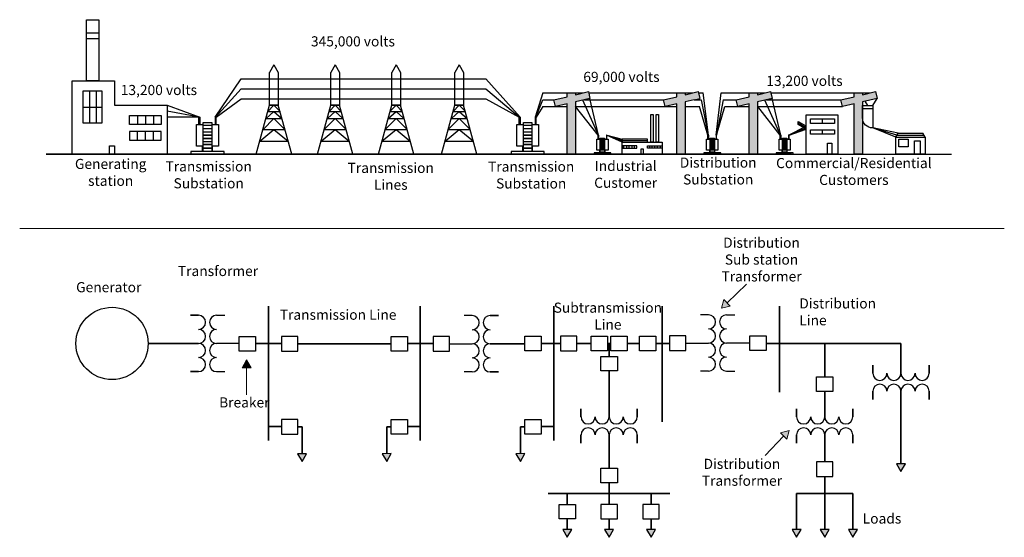
# Model space of a CAD drawing. Units: millimetres. Extents: x 50.7 to 99.4, y 24.2 to 49.8.
import ezdxf

# ---------------------------------------------------------------- set-up
doc = ezdxf.new("R2010")
doc.units = ezdxf.units.MM
doc.header["$MEASUREMENT"] = 0
for name, color, linetype, lineweight in [('E-ANNO-PATT', 8, 'Continuous', 13), ('E-ANNO-SYMB', 2, 'Continuous', 18), ('E-ANNO-TEXT', 7, 'Continuous', 25), ('E-ONEL-DEVC', 4, 'Continuous', 25), ('E-ONEL-LINE', 7, 'Continuous', 35), ('E-PICT', 7, 'Continuous', 25), ('E-PICT-GRND', 8, 'Continuous', 35)]:
    doc.layers.add(name, color=color, linetype=linetype, lineweight=lineweight)
doc.styles.get("Standard").update_dxf_attribs({"font": 'arial.ttf'})

# ---------------------------------------------------------------- blocks, each defined once
blk = doc.blocks.new('TRANSMISSION-TOWER')
for p, q in [((0.869, 4.42), (0.654, 4.049)), ((0.869, 4.42), (1.083, 4.049)), ((-0.005, 0.004), (0.654, 2.432)), ((0.485, 1.767), (0.869, 2.12)), ((0.57, 2.12), (0.869, 2.432)), ((0.57, 2.12), (1.168, 2.12)), ((0.654, 2.432), (1.083, 2.432)), ((0.869, 2.432), (1.168, 2.12)), ((0.869, 2.12), (1.252, 1.767)), ((1.743, 0.004), (1.083, 2.432)), ((0.325, 1.218), (0.869, 1.767)), ((0.869, 1.767), (1.413, 1.218)), ((0.171, 0.651), (0.869, 1.218)), ((0.325, 1.218), (1.413, 1.218)), ((0.869, 1.218), (1.567, 0.651)), ((0.171, 0.651), (1.567, 0.651))]:
    blk.add_line(p, q)
for points in [[(1.083, 4.049), (1.083, 2.432), (0.654, 2.432), (0.654, 4.049)], [(0.485, 1.767), (1.252, 1.767)]]:
    blk.add_lwpolyline(points)
blk = doc.blocks.new('DIST-POLE')
for points in [[(0.648, 2.843), (0.648, 3.03), (1.066, 3.03), (1.066, 2.942)], [(1.066, 2.942), (1.705, 3.093), (1.784, 2.759), (1.066, 2.589)], [(0.648, 2.49), (0.079, 2.355), (0, 2.689), (0.648, 2.843)], [(1.066, 2.589), (1.066, 0), (0.648, 0), (0.648, 2.49)]]:
    blk.add_lwpolyline(points)
blk = doc.blocks.new('TRANSFORMER-SYM')
for p, q in [((0.348, 2.786), (0.751, 2.786)), ((1.469, 1.393), (0.348, 1.393)), ((0.348, 0), (0.751, 0))]:
    blk.add_line(p, q)
for centre in [(0.348, 2.437), (0.348, 1.741), (0.348, 1.045), (0.348, 0.349)]:
    blk.add_arc(centre, 0.348, 90, 270)
blk = doc.blocks.new('BREAKER-SYM')
blk.add_lwpolyline([(0, 0.721), (0.81, 0.721), (0.81, 0), (0, 0)], close=True)
blk = doc.blocks.new('GROUND-ARROW')
blk.add_lwpolyline([(0, 0.385), (0.223, 0), (0.445, 0.385)], close=True)

msp = doc.modelspace()

# ---------------------------------------------------------------- hatches: boundary and pattern name
at = {"layer": 'E-ANNO-PATT'}
h = msp.add_hatch(color=256, dxfattribs=at)
h.dxf.hatch_style = 1
h.paths.add_polyline_path([(78.15, 45.743), (78.868, 45.913), (78.789, 46.247), (78.15, 46.096), (78.15, 46.184), (77.732, 46.184), (77.732, 45.997), (77.084, 45.843), (77.163, 45.509), (77.732, 45.644), (77.732, 43.154), (78.15, 43.154)])
h.paths.add_polyline_path([(83.579, 45.743), (84.017, 45.847), (84.297, 45.913), (84.217, 46.247), (83.579, 46.096), (83.579, 46.184), (83.16, 46.184), (83.16, 45.997), (82.512, 45.843), (82.591, 45.509), (83.16, 45.644), (83.16, 43.154), (83.579, 43.154)])
h.paths.add_polyline_path([(87.162, 45.743), (87.88, 45.913), (87.8, 46.247), (87.162, 46.096), (87.162, 46.184), (86.743, 46.184), (86.743, 45.997), (86.095, 45.843), (86.174, 45.509), (86.743, 45.644), (86.743, 43.154), (87.162, 43.154)])
h.paths.add_polyline_path([(92.348, 45.743), (93.065, 45.913), (92.986, 46.247), (92.348, 46.096), (92.348, 46.184), (91.929, 46.184), (91.929, 45.997), (91.281, 45.843), (91.36, 45.509), (91.929, 45.644), (91.929, 43.154), (92.348, 43.154)])
h.paths.add_polyline_path([(69.038, 28.346), (68.593, 28.346), (68.816, 27.961)])
h.paths.add_polyline_path([(64.848, 28.346), (64.403, 28.346), (64.626, 27.961)])
h.paths.add_polyline_path([(75.652, 28.346), (75.207, 28.346), (75.429, 27.961)])
h.paths.add_polyline_path([(77.968, 24.596), (77.523, 24.596), (77.745, 24.211)])
h.paths.add_polyline_path([(80.039, 24.596), (79.594, 24.596), (79.816, 24.211)])
h.paths.add_polyline_path([(82.109, 24.596), (81.664, 24.596), (81.887, 24.211)])
h.paths.add_polyline_path([(89.309, 24.596), (88.864, 24.596), (89.086, 24.211)])
h.paths.add_polyline_path([(90.702, 24.596), (90.257, 24.596), (90.479, 24.211)])
h.paths.add_polyline_path([(92.094, 24.596), (91.649, 24.596), (91.872, 24.211)])
h.paths.add_polyline_path([(94.472, 27.842), (94.027, 27.842), (94.249, 27.457)])
h.paths.add_polyline_path([(88.712, 29.497), (88.286, 29.37), (88.609, 29.064)])
h.paths.add_polyline_path([(85.496, 35.962), (85.371, 35.535), (85.803, 35.64)])
h = msp.add_hatch(color=256, dxfattribs=at)
h.dxf.hatch_style = 1
h.paths.add_polyline_path([(62.106, 32.593), (61.884, 32.979), (61.661, 32.593)])

# ---------------------------------------------------------------- linework, layer by layer
at = {"layer": 'E-ANNO-SYMB'}
for p, q in [((50.661, 39.486), (99.361, 39.486)), ((86.614, 36.72), (85.649, 35.801)), ((61.884, 31.261), (61.884, 32.593)), ((87.532, 28.25), (88.447, 29.217))]:
    msp.add_line(p, q, dxfattribs=at)
for points in [[(85.803, 35.64), (85.371, 35.535), (85.496, 35.962)], [(61.661, 32.593), (61.884, 32.979), (62.106, 32.593)], [(88.286, 29.37), (88.712, 29.497), (88.609, 29.064)]]:
    msp.add_lwpolyline(points, close=True, dxfattribs=at)
at = {"layer": 'E-ONEL-DEVC'}
for points in [[(83.613, 34.176), (82.803, 34.176), (82.803, 33.455), (83.613, 33.455)], [(83.613, 34.176), (82.803, 34.176), (82.803, 33.455), (83.613, 33.455)], [(86.779, 34.176), (87.588, 34.176), (87.588, 33.455), (86.779, 33.455)], [(86.779, 34.176), (87.588, 34.176), (87.588, 33.455), (86.779, 33.455)]]:
    msp.add_lwpolyline(points, close=True, dxfattribs=at)
msp.add_circle((55.229, 33.796), 1.787, dxfattribs=at)
for centre, start, end in [((59.508, 34.84), 270, 90), ((73.933, 34.825), 90, 270), ((59.508, 34.144), 270, 90), ((73.933, 34.129), 90, 270), ((59.508, 33.448), 270, 90), ((73.933, 33.432), 90, 270), ((59.508, 32.752), 270, 90), ((73.933, 32.736), 90, 270), ((93.205, 32.319), 180, 0), ((93.901, 32.319), 180, 0), ((94.597, 32.319), 180, 0), ((95.294, 32.319), 180, 0), ((93.205, 31.431), 0, 180), ((93.901, 31.431), 0, 180), ((94.597, 31.431), 0, 180), ((95.294, 31.431), 0, 180), ((78.772, 30.164), 180, 0), ((79.468, 30.164), 180, 0), ((80.164, 30.164), 180, 0), ((80.86, 30.164), 180, 0), ((89.435, 30.164), 180, 0), ((90.131, 30.164), 180, 0), ((90.827, 30.164), 180, 0), ((91.523, 30.164), 180, 0), ((78.772, 29.275), 0, 180), ((79.468, 29.275), 0, 180), ((80.164, 29.275), 0, 180), ((80.86, 29.275), 0, 180), ((89.435, 29.275), 0, 180), ((90.131, 29.275), 0, 180), ((90.827, 29.275), 0, 180), ((91.523, 29.275), 0, 180)]:
    msp.add_arc(centre, 0.348, start, end, dxfattribs=at)
at = {"layer": 'E-ONEL-LINE'}
for p, q in [((62.967, 35.636), (62.967, 28.998)), ((70.475, 35.636), (70.475, 28.998)), ((77.088, 35.636), (77.088, 28.998)), ((82.442, 35.636), (82.442, 29.925)), ((88.248, 35.636), (88.248, 31.386)), ((59.508, 35.189), (59.106, 35.189)), ((73.933, 35.173), (74.336, 35.173)), ((57.266, 33.796), (57.017, 33.796)), ((57.266, 33.796), (59.508, 33.796)), ((62.967, 33.796), (62.328, 33.796)), ((62.967, 33.796), (63.606, 33.796)), ((64.416, 33.78), (69.026, 33.78)), ((70.475, 33.796), (69.836, 33.796)), ((70.475, 33.796), (71.113, 33.796)), ((75.055, 33.78), (73.933, 33.78)), ((75.055, 33.78), (75.64, 33.78)), ((77.088, 33.796), (76.449, 33.796)), ((77.088, 33.796), (77.408, 33.796)), ((78.217, 33.796), (78.926, 33.796)), ((79.736, 33.796), (79.896, 33.796)), ((79.816, 33.796), (79.816, 33.158)), ((81.312, 33.796), (80.706, 33.796)), ((82.122, 33.796), (82.803, 33.796)), ((88.269, 33.796), (87.588, 33.796)), ((88.248, 33.796), (94.249, 33.796)), ((90.479, 33.796), (90.479, 32.147)), ((94.249, 33.796), (94.249, 32.319)), ((92.857, 32.319), (92.857, 32.722)), ((95.642, 32.319), (95.642, 32.722)), ((59.508, 32.403), (59.106, 32.403)), ((73.933, 32.388), (74.336, 32.388)), ((79.816, 32.437), (79.816, 30.164)), ((90.479, 31.426), (90.479, 30.164)), ((92.857, 31.431), (92.857, 31.028)), ((94.249, 31.431), (94.249, 30.843)), ((95.642, 31.431), (95.642, 31.028)), ((94.249, 30.843), (94.249, 27.842)), ((78.423, 30.164), (78.423, 30.567)), ((81.209, 30.164), (81.209, 30.567)), ((89.086, 30.164), (89.086, 30.567)), ((91.872, 30.164), (91.872, 30.567)), ((62.967, 29.694), (63.606, 29.694)), ((64.416, 29.678), (64.626, 29.678)), ((64.626, 29.678), (64.626, 28.346)), ((69.026, 29.678), (68.816, 29.678)), ((68.816, 29.678), (68.816, 28.346)), ((70.475, 29.694), (69.836, 29.694)), ((75.64, 29.678), (75.429, 29.678)), ((75.429, 29.678), (75.429, 28.346)), ((77.088, 29.694), (76.449, 29.694)), ((78.423, 29.275), (78.423, 28.872)), ((79.816, 29.275), (79.816, 27.626)), ((81.209, 29.275), (81.209, 28.872)), ((89.086, 29.275), (89.086, 28.872)), ((90.479, 29.197), (90.479, 29.275)), ((91.872, 29.275), (91.872, 28.872)), ((90.479, 27.936), (90.479, 29.197)), ((79.816, 26.905), (79.816, 25.84)), ((90.479, 27.214), (90.479, 24.596)), ((79.816, 26.372), (76.807, 26.372)), ((77.745, 25.84), (77.745, 26.372)), ((79.816, 26.372), (82.825, 26.372)), ((81.887, 25.84), (81.887, 26.372)), ((89.086, 26.372), (91.872, 26.372)), ((89.086, 26.372), (89.086, 24.596)), ((91.872, 26.372), (91.872, 24.596)), ((77.745, 25.119), (77.745, 24.596)), ((79.816, 25.119), (79.816, 24.596)), ((81.887, 25.119), (81.887, 24.596))]:
    msp.add_line(p, q, dxfattribs=at)
at = {"layer": 'E-PICT'}
for p, q in [((53.97, 49.151), (54.583, 49.151)), ((54.583, 48.854), (53.97, 48.854)), ((60.324, 44.984), (61.609, 46.882)), ((61.609, 46.882), (73.25, 46.882)), ((73.25, 46.882), (73.717, 46.882)), ((73.717, 46.882), (75.407, 44.984)), ((54.111, 46.29), (54.111, 44.682)), ((54.443, 46.29), (54.443, 44.682)), ((60.349, 44.984), (61.609, 46.39)), ((61.609, 46.39), (73.25, 46.39)), ((73.25, 46.39), (73.717, 46.39)), ((73.717, 46.39), (75.382, 44.984)), ((60.374, 44.984), (61.609, 45.883)), ((61.609, 45.883), (73.25, 45.883)), ((73.25, 45.883), (73.717, 45.883)), ((73.717, 45.883), (75.357, 44.984)), ((76.543, 46.184), (76.157, 44.984)), ((76.182, 44.984), (76.543, 45.847)), ((76.543, 46.184), (78.523, 46.184)), ((76.543, 45.847), (77.097, 45.847)), ((79.282, 44.086), (78.509, 45.828)), ((78.589, 45.847), (82.526, 45.847)), ((78.804, 46.184), (83.952, 46.184)), ((79.295, 44.086), (78.868, 45.913)), ((84.017, 45.847), (84.297, 45.913)), ((84.017, 45.847), (84.366, 45.847)), ((84.232, 46.184), (84.474, 46.184)), ((84.366, 45.847), (84.711, 44.086)), ((84.724, 44.086), (84.474, 46.184)), ((85.105, 44.086), (85.355, 46.184)), ((85.462, 45.847), (85.118, 44.086)), ((85.355, 46.184), (85.587, 46.184)), ((85.462, 45.847), (85.587, 45.847)), ((85.587, 46.184), (85.709, 46.184)), ((85.587, 45.847), (85.709, 45.847)), ((85.709, 46.184), (87.535, 46.184)), ((85.709, 45.847), (86.109, 45.847)), ((88.294, 44.086), (87.521, 45.828)), ((87.6, 45.847), (91.294, 45.847)), ((87.815, 46.184), (92.72, 46.184)), ((88.307, 44.086), (87.88, 45.913)), ((92.864, 45.554), (93.065, 45.913)), ((53.802, 45.486), (54.73, 45.486)), ((57.951, 45.582), (59.574, 44.984)), ((76.543, 45.509), (76.207, 44.984)), ((76.543, 45.509), (77.732, 45.509)), ((78.15, 45.509), (83.16, 45.509)), ((79.27, 44.086), (78.15, 45.509)), ((83.579, 45.509), (84.289, 45.509)), ((84.698, 44.086), (84.289, 45.509)), ((85.131, 44.086), (85.54, 45.509)), ((85.54, 45.509), (85.587, 45.509)), ((85.587, 45.509), (85.786, 45.509)), ((85.786, 45.509), (86.743, 45.509)), ((88.281, 44.086), (87.162, 45.509)), ((87.162, 45.509), (91.36, 45.509)), ((92.864, 45.392), (92.348, 45.392)), ((92.606, 45.554), (92.479, 45.774)), ((56.483, 45.063), (56.483, 44.623)), ((56.877, 45.063), (56.877, 44.623)), ((57.271, 45.063), (57.271, 44.623)), ((59.549, 44.984), (57.951, 45.277)), ((59.524, 44.984), (57.951, 44.984)), ((90.366, 44.667), (90.366, 44.896)), ((59.739, 44.592), (60.159, 44.592)), ((60.159, 44.571), (59.739, 44.571)), ((59.739, 44.424), (60.159, 44.424)), ((60.159, 44.403), (59.739, 44.403)), ((75.572, 44.592), (75.992, 44.592)), ((75.992, 44.571), (75.572, 44.571)), ((75.572, 44.424), (75.992, 44.424)), ((75.992, 44.403), (75.572, 44.403)), ((88.688, 44.086), (89.555, 44.544)), ((88.701, 44.086), (89.555, 44.464)), ((88.714, 44.086), (89.555, 44.384)), ((89.159, 44.613), (89.159, 44.772)), ((89.159, 44.772), (89.214, 44.739)), ((89.555, 44.464), (89.159, 44.692)), ((89.555, 44.384), (89.159, 44.613)), ((89.555, 44.544), (89.214, 44.741)), ((90.366, 44.135), (90.366, 44.364)), ((94.045, 44.093), (92.848, 44.448)), ((93.988, 43.994), (92.864, 44.448)), ((94.103, 44.192), (92.864, 44.448)), ((56.483, 43.843), (56.483, 44.283)), ((56.877, 43.843), (56.877, 44.283)), ((57.271, 43.843), (57.271, 44.283)), ((59.739, 44.262), (60.159, 44.262)), ((60.159, 44.241), (59.739, 44.241)), ((59.739, 44.102), (60.159, 44.102)), ((60.159, 44.081), (59.739, 44.081)), ((59.739, 43.938), (60.159, 43.938)), ((60.159, 43.917), (59.739, 43.917)), ((75.572, 44.262), (75.992, 44.262)), ((75.992, 44.241), (75.572, 44.241)), ((75.572, 44.102), (75.992, 44.102)), ((75.992, 44.081), (75.572, 44.081)), ((75.572, 43.938), (75.992, 43.938)), ((75.992, 43.917), (75.572, 43.917)), ((79.379, 43.886), (79.593, 43.886)), ((79.593, 43.876), (79.379, 43.876)), ((80.452, 43.743), (79.677, 44.086)), ((79.69, 44.086), (80.452, 43.822)), ((79.703, 44.086), (80.452, 43.9)), ((84.808, 43.886), (85.021, 43.886)), ((85.021, 43.876), (84.808, 43.876)), ((88.391, 43.886), (88.604, 43.886)), ((88.604, 43.876), (88.391, 43.876)), ((93.988, 43.994), (94.103, 44.192)), ((94.045, 44.093), (95.385, 44.093)), ((94.103, 44.192), (95.328, 44.192)), ((95.442, 43.994), (95.328, 44.192)), ((59.708, 43.284), (59.708, 43.544)), ((59.739, 43.784), (60.159, 43.784)), ((60.159, 43.763), (59.739, 43.763)), ((59.739, 43.641), (60.159, 43.641)), ((60.159, 43.62), (59.739, 43.62)), ((59.739, 43.461), (60.159, 43.461)), ((60.159, 43.44), (59.739, 43.44)), ((60.198, 43.284), (60.198, 43.544)), ((75.54, 43.284), (75.54, 43.544)), ((75.572, 43.784), (75.992, 43.784)), ((75.992, 43.763), (75.572, 43.763)), ((75.572, 43.641), (75.992, 43.641)), ((75.992, 43.62), (75.572, 43.62)), ((75.572, 43.461), (75.992, 43.461)), ((75.992, 43.44), (75.572, 43.44)), ((76.03, 43.284), (76.03, 43.544)), ((79.363, 43.22), (79.363, 43.353)), ((79.379, 43.801), (79.593, 43.801)), ((79.593, 43.79), (79.379, 43.79)), ((79.379, 43.719), (79.593, 43.719)), ((79.593, 43.708), (79.379, 43.708)), ((79.379, 43.637), (79.593, 43.637)), ((79.593, 43.626), (79.379, 43.626)), ((79.379, 43.553), (79.593, 43.553)), ((79.593, 43.542), (79.379, 43.542)), ((79.379, 43.475), (79.593, 43.475)), ((79.593, 43.464), (79.379, 43.464)), ((79.379, 43.402), (79.593, 43.402)), ((79.593, 43.392), (79.379, 43.392)), ((79.613, 43.22), (79.613, 43.353)), ((80.452, 43.822), (81.714, 43.822)), ((80.543, 43.449), (80.543, 43.564)), ((80.683, 43.449), (80.683, 43.564)), ((80.814, 43.449), (80.814, 43.564)), ((80.948, 43.449), (80.948, 43.564)), ((81.069, 43.449), (81.069, 43.564)), ((81.824, 43.449), (81.824, 43.564)), ((81.945, 43.449), (81.945, 43.564)), ((82.079, 43.449), (82.079, 43.564)), ((82.21, 43.449), (82.21, 43.564)), ((82.35, 43.449), (82.35, 43.564)), ((84.791, 43.22), (84.791, 43.353)), ((84.808, 43.801), (85.021, 43.801)), ((85.021, 43.79), (84.808, 43.79)), ((84.808, 43.719), (85.021, 43.719)), ((85.021, 43.708), (84.808, 43.708)), ((84.808, 43.637), (85.021, 43.637)), ((85.021, 43.626), (84.808, 43.626)), ((84.808, 43.553), (85.021, 43.553)), ((85.021, 43.542), (84.808, 43.542)), ((84.808, 43.475), (85.021, 43.475)), ((85.021, 43.464), (84.808, 43.464)), ((84.808, 43.402), (85.021, 43.402)), ((85.021, 43.392), (84.808, 43.392)), ((85.041, 43.22), (85.041, 43.353)), ((88.374, 43.22), (88.374, 43.353)), ((88.391, 43.801), (88.604, 43.801)), ((88.604, 43.79), (88.391, 43.79)), ((88.391, 43.719), (88.604, 43.719)), ((88.604, 43.708), (88.391, 43.708)), ((88.391, 43.637), (88.604, 43.637)), ((88.604, 43.626), (88.391, 43.626)), ((88.391, 43.553), (88.604, 43.553)), ((88.604, 43.542), (88.391, 43.542)), ((88.391, 43.475), (88.604, 43.475)), ((88.604, 43.464), (88.391, 43.464)), ((88.391, 43.402), (88.604, 43.402)), ((88.604, 43.392), (88.391, 43.392)), ((88.624, 43.22), (88.624, 43.353)), ((79.379, 43.311), (79.593, 43.311)), ((79.593, 43.3), (79.379, 43.3)), ((84.808, 43.311), (85.021, 43.311)), ((85.021, 43.3), (84.808, 43.3)), ((88.391, 43.311), (88.604, 43.311)), ((88.604, 43.3), (88.391, 43.3)), ((88.827, 43.154), (96.751, 43.154))]:
    msp.add_line(p, q, dxfattribs=at)
for points in [[(54.583, 46.778), (53.97, 46.778), (53.97, 49.803), (54.583, 49.803)], [(53.802, 46.29), (54.73, 46.29), (54.73, 44.682), (53.802, 44.682)], [(56.089, 45.063), (57.665, 45.063), (57.665, 44.623), (56.089, 44.623)], [(59.574, 44.623), (59.524, 44.623), (59.524, 44.984), (59.574, 44.984)], [(60.324, 44.623), (60.374, 44.623), (60.374, 44.984), (60.324, 44.984)], [(75.407, 44.623), (75.357, 44.623), (75.357, 44.984), (75.407, 44.984)], [(76.157, 44.623), (76.207, 44.623), (76.207, 44.984), (76.157, 44.984)], [(81.877, 45.114), (81.986, 45.114), (81.986, 43.743), (81.877, 43.743)], [(82.143, 45.114), (82.252, 45.114), (82.252, 43.743), (82.143, 43.743)], [(89.555, 45.106), (91.121, 45.106), (91.121, 43.154), (89.555, 43.154)], [(89.77, 44.896), (90.962, 44.896), (90.962, 44.667), (89.77, 44.667)], [(89.77, 44.364), (90.962, 44.364), (90.962, 44.135), (89.77, 44.135)], [(56.089, 43.843), (57.665, 43.843), (57.665, 44.283), (56.089, 44.283)], [(79.295, 43.902), (79.27, 43.902), (79.27, 44.086), (79.295, 44.086)], [(79.677, 43.902), (79.703, 43.902), (79.703, 44.086), (79.677, 44.086)], [(80.452, 43.743), (81.714, 43.743), (81.714, 43.9), (80.452, 43.9)], [(84.724, 43.902), (84.698, 43.902), (84.698, 44.086), (84.724, 44.086)], [(85.105, 43.902), (85.131, 43.902), (85.131, 44.086), (85.105, 44.086)], [(88.307, 43.902), (88.281, 43.902), (88.281, 44.086), (88.307, 44.086)], [(88.688, 43.902), (88.714, 43.902), (88.714, 44.086), (88.688, 44.086)], [(93.988, 43.994), (95.442, 43.994), (95.442, 43.154), (93.988, 43.154)], [(94.143, 43.897), (94.601, 43.897), (94.601, 43.518), (94.143, 43.518)], [(55.349, 43.154), (55.11, 43.154), (55.11, 43.569), (55.349, 43.569)], [(80.452, 43.743), (82.442, 43.743), (82.442, 43.154), (80.452, 43.154)], [(80.452, 43.449), (81.177, 43.449), (81.177, 43.564), (80.452, 43.564)], [(81.495, 43.154), (81.399, 43.154), (81.399, 43.415), (81.495, 43.415)], [(82.442, 43.449), (81.716, 43.449), (81.716, 43.564), (82.442, 43.564)], [(90.617, 43.693), (90.831, 43.693), (90.831, 43.154), (90.617, 43.154)], [(94.923, 43.818), (95.194, 43.818), (95.194, 43.154), (94.923, 43.154)], [(59.132, 43.154), (60.773, 43.154), (60.773, 43.284), (59.132, 43.284)], [(74.965, 43.154), (76.606, 43.154), (76.606, 43.284), (74.965, 43.284)], [(79.07, 43.154), (79.906, 43.154), (79.906, 43.22), (79.07, 43.22)], [(84.498, 43.154), (85.334, 43.154), (85.334, 43.22), (84.498, 43.22)], [(88.081, 43.154), (88.917, 43.154), (88.917, 43.22), (88.081, 43.22)]]:
    msp.add_lwpolyline(points, close=True, dxfattribs=at)
for points in [[(55.349, 43.154), (53.257, 43.154), (53.257, 46.778), (55.349, 46.778), (55.349, 45.582)], [(83.16, 45.644), (82.591, 45.509), (82.512, 45.843), (83.16, 45.997)], [(83.16, 45.997), (83.16, 46.184), (83.579, 46.184), (83.579, 46.096)], [(83.579, 46.096), (84.217, 46.247), (84.297, 45.913)], [(84.017, 45.847), (83.579, 45.743)], [(55.349, 45.582), (57.951, 45.582), (57.951, 43.154), (55.349, 43.154)], [(83.579, 45.743), (83.579, 43.154), (83.16, 43.154), (83.16, 45.644)], [(59.739, 43.544), (59.409, 43.544), (59.409, 44.623), (59.739, 44.623)], [(59.739, 43.284), (59.739, 44.717), (60.159, 44.717), (60.159, 43.284)], [(60.159, 44.623), (60.489, 44.623), (60.489, 43.544), (60.159, 43.544)], [(75.572, 43.544), (75.242, 43.544), (75.242, 44.623), (75.572, 44.623)], [(75.572, 43.284), (75.572, 44.717), (75.992, 44.717), (75.992, 43.284)], [(75.992, 44.623), (76.322, 44.623), (76.322, 43.544), (75.992, 43.544)], [(79.379, 43.353), (79.211, 43.353), (79.211, 43.902), (79.379, 43.902)], [(79.379, 43.22), (79.379, 43.95), (79.593, 43.95), (79.593, 43.22)], [(79.593, 43.902), (79.761, 43.902), (79.761, 43.353), (79.593, 43.353)], [(84.808, 43.353), (84.639, 43.353), (84.639, 43.902), (84.808, 43.902)], [(84.808, 43.22), (84.808, 43.95), (85.021, 43.95), (85.021, 43.22)], [(85.021, 43.902), (85.19, 43.902), (85.19, 43.353), (85.021, 43.353)], [(88.391, 43.353), (88.222, 43.353), (88.222, 43.902), (88.391, 43.902)], [(88.391, 43.22), (88.391, 43.95), (88.604, 43.95), (88.604, 43.22)], [(88.604, 43.902), (88.773, 43.902), (88.773, 43.353), (88.604, 43.353)]]:
    msp.add_lwpolyline(points, dxfattribs=at)
msp.add_lwpolyline([(92.348, 45.554), (92.864, 45.554), (92.864, 44.448), (92.848, 44.448, -0.414214), (92.348, 44.948)], format="xyb", close=True, dxfattribs=at)
at = {"layer": 'E-PICT-GRND'}
msp.add_line((51.964, 43.154), (88.827, 43.154), dxfattribs=at)

# ---------------------------------------------------------------- block references
at = {"layer": 'E-ONEL-DEVC'}
for name, p in [('TRANSFORMER-SYM', (60.049, 32.403)), ('TRANSFORMER-SYM', (85.275, 32.423)), ('BREAKER-SYM', (61.518, 33.42)), ('BREAKER-SYM', (69.026, 33.42)), ('BREAKER-SYM', (75.639, 33.435)), ('BREAKER-SYM', (78.925, 33.435)), ('BREAKER-SYM', (79.896, 33.435)), ('BREAKER-SYM', (81.312, 33.435)), ('BREAKER-SYM', (79.411, 32.437)), ('BREAKER-SYM', (90.074, 31.426)), ('BREAKER-SYM', (69.026, 29.318)), ('BREAKER-SYM', (75.639, 29.318)), ('GROUND-ARROW', (64.403, 27.961)), ('BREAKER-SYM', (79.411, 26.905)), ('BREAKER-SYM', (77.34, 25.119))]:
    msp.add_blockref(name, p, dxfattribs=at)
for name, p, rotation in [('TRANSFORMER-SYM', (73.393, 35.173), 180), ('TRANSFORMER-SYM', (85.082, 35.208), 180), ('GROUND-ARROW', (68.705, 28.539), 239.9999999999986), ('GROUND-ARROW', (75.319, 28.539), 239.9999999999986), ('GROUND-ARROW', (94.139, 28.035), 239.9999999999984), ('GROUND-ARROW', (77.634, 24.789), 239.9999999999999), ('GROUND-ARROW', (79.705, 24.789), 239.9999999999995), ('GROUND-ARROW', (81.776, 24.789), 240.0000000000009), ('GROUND-ARROW', (88.976, 24.789), 240.0000000000011), ('GROUND-ARROW', (90.368, 24.789), 239.9999999999993), ('GROUND-ARROW', (91.761, 24.789), 240.0000000000002)]:
    msp.add_blockref(name, p, dxfattribs=dict(at, rotation=rotation))
at = {"layer": 'E-ONEL-DEVC', "extrusion": (0, 0, -1), "zscale": -1}
for p in [(-64.416, 33.42), (-71.924, 33.42), (-78.218, 33.435), (-64.416, 29.318), (-80.221, 25.119), (-82.292, 25.119)]:
    msp.add_blockref('BREAKER-SYM', p, dxfattribs=at)
at = {"layer": 'E-ONEL-DEVC', "extrusion": (0, 0, -1), "zscale": -1, "rotation": 180}
msp.add_blockref('BREAKER-SYM', (-90.074, 27.935), dxfattribs=at)
at = {"layer": 'E-PICT'}
for name, p in [('TRANSMISSION-TOWER', (62.37, 43.15)), ('TRANSMISSION-TOWER', (65.398, 43.15)), ('TRANSMISSION-TOWER', (68.405, 43.15)), ('TRANSMISSION-TOWER', (71.535, 43.15)), ('DIST-POLE', (77.084, 43.154)), ('DIST-POLE', (86.095, 43.154)), ('DIST-POLE', (91.281, 43.154))]:
    msp.add_blockref(name, p, dxfattribs=at)

# ---------------------------------------------------------------- texts
at = {"layer": 'E-ANNO-TEXT', "char_height": 0.5, "attachment_point": 1}
for s, width, heights, insert in [('345,000 volts', 4.65187, [0], (65.067, 48.982)), ('69,000 volts', 4.65187, [0], (78.537, 47.226)), ('13,200 volts', 4.65187, [0], (87.591, 47.03)), ('13,200 volts', 4.65187, [0], (55.659, 46.577)), ('\\pxqc;Generating\\Pstation', 4.65187, [0], (52.836, 42.922)), ('\\pxqc;Industrial\\PCustomer', 4.65187, [0], (78.306, 42.824)), ('\\pxqc;Distribution Substation', 4.65187, [0], (82.883, 42.989)), ('\\pxqc;Commercial/Residential\\PCustomers', 4.65187, [0], (89.593, 42.964)), ('\\pxqc;Transmission\\PSubstation', 4.65187, [0], (57.682, 42.798)), ('\\pxqc;Transmission\\PLines', 4.65187, [0], (66.687, 42.727)), ('\\pxqc;Transmission\\PSubstation', 4.65187, [0], (73.633, 42.79)), ('\\pxqc;Distribution\\PSub station\\PTransformer', 4.65187, [0], (85.026, 39.027)), ('Transformer', 4.65187, [0], (58.485, 37.628)), ('Generator', 4.65187, [0], (53.451, 36.827)), ('Distribution Line', 5.24295, [0.961], (89.221, 36.025)), ('\\pxqc;Subtransmission\\PLine', 4.65187, [0], (77.425, 35.815)), ('Transmission Line', 5.84574, [1.4], (63.523, 35.467)), ('Breaker', 4.65187, [0], (60.524, 31.129)), ('\\pxqc;Distribution\\PTransformer', 4.65187, [0], (84.057, 28.092)), ('Loads', 4.65187, [0], (92.357, 25.389))]:
    msp.add_mtext_dynamic_manual_height_columns(s, width=width, gutter_width=1, heights=heights, dxfattribs=dict(at, insert=insert))

doc.saveas('drawing.dxf')
